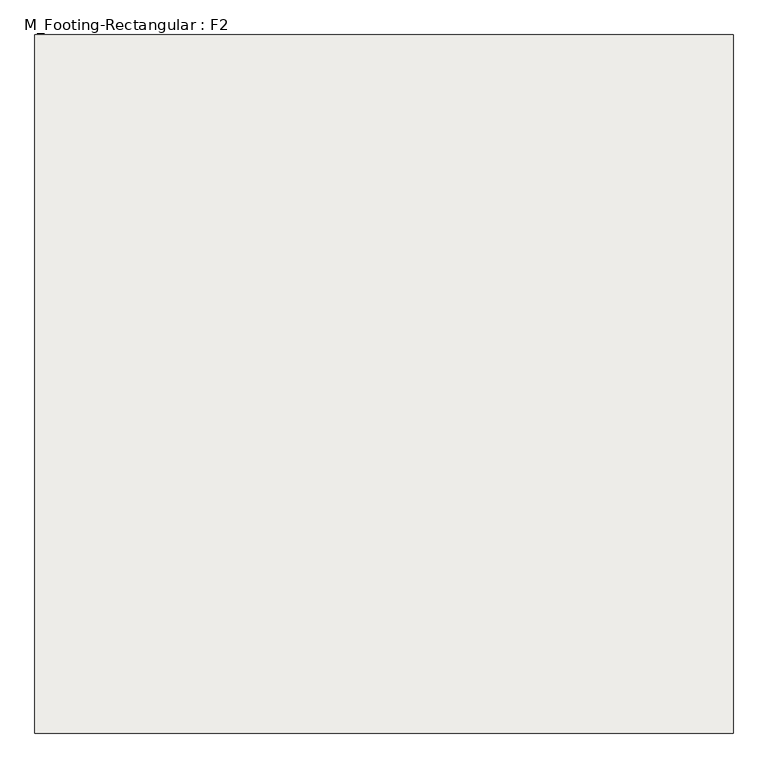
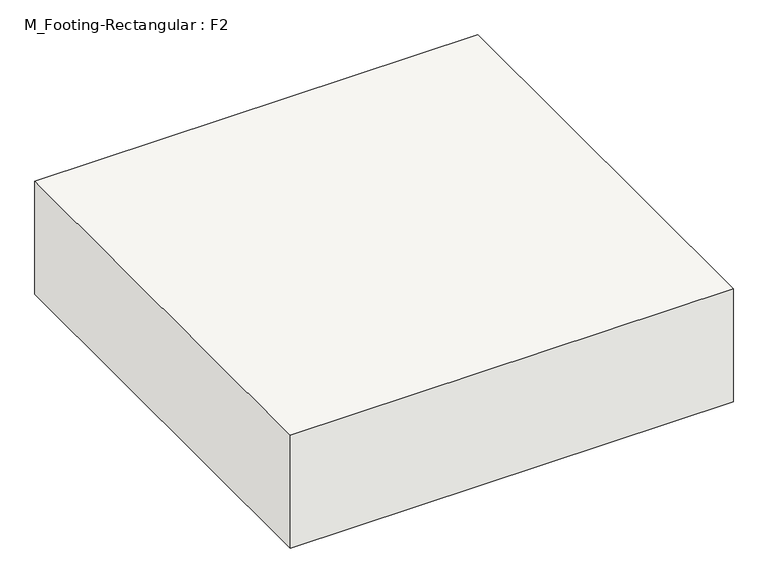
"""IFC4 building model written with IfcOpenShell, lengths in millimetres: slab geometry, M_Footing-Rectangular : F2."""

from ifc_helpers import new_model, si_unit, frame, origin, place, context, project, spatial, polyline, outline, extrude, source, transform, mapped, element, save


def m_footing_rectangular_f2_e38db0b8(model_context):
    return source(origin(), model_context, "Body", "SweptSolid", [
        extrude(outline(polyline([(990.6, 990.6), (990.6, -990.6), (-990.6, -990.6), (-990.6, 990.6), (990.6, 990.6)])), frame((0.0, 0.0, -533.4), z_axis=(0.0, 0.0, 1.0), x_axis=(1.0, 0.0, 0.0)), (0.0, 0.0, 1.0), 533.4),
    ])


if __name__ == "__main__":
    model = new_model("IFC4")
    model_context = context("Model", 3, world=origin())
    ifc_project = project(units=[si_unit("LENGTHUNIT", "METRE", prefix="MILLI")], contexts=[model_context])
    site = spatial("IfcSite", under=ifc_project)
    building = spatial("IfcBuilding", under=site)
    placement = place(None, origin())
    m_footing_rectangular_f2_shape = m_footing_rectangular_f2_e38db0b8(model_context)
    element("IfcSlab", 1, ObjectType="M_Footing-Rectangular : F2", at=placement, inside=building, context=model_context, shape_type="MappedRepresentation", body=[
        mapped(m_footing_rectangular_f2_shape, transform((0.0, 0.0, 0.0), x_axis=(1.0, 0.0, 0.0), y_axis=(0.0, 1.0, 0.0), z_axis=(0.0, 0.0, 1.0))),
    ])
    save(model, "model.ifc")

# Revit data of these elements
# Type "M_Footing-Rectangular : F2"
#   Width = 1981.2 mm
#   Length = 1981.2 mm
#   Foundation Thickness = 533.4 mm
#   Structural Material [instance default] = Concrete, Cast-in-Place gray
#   Assembly Code = ""
# Element 1 (IfcSlab, "M_Footing-Rectangular : F2")
#   Materials on its faces: "Concrete, Cast-in-Place gray"
# Materials
#   "Concrete, Cast-in-Place gray": class "Concrete", colour RGB 192 192 192, transparency 0, Description = "Cast-in-place concrete", Cost = 0
